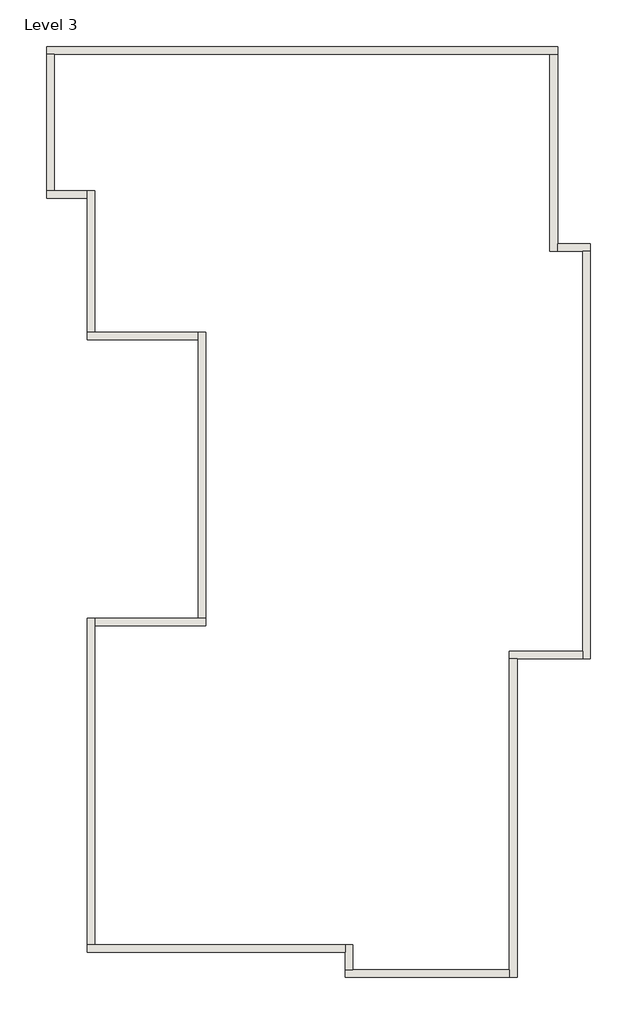
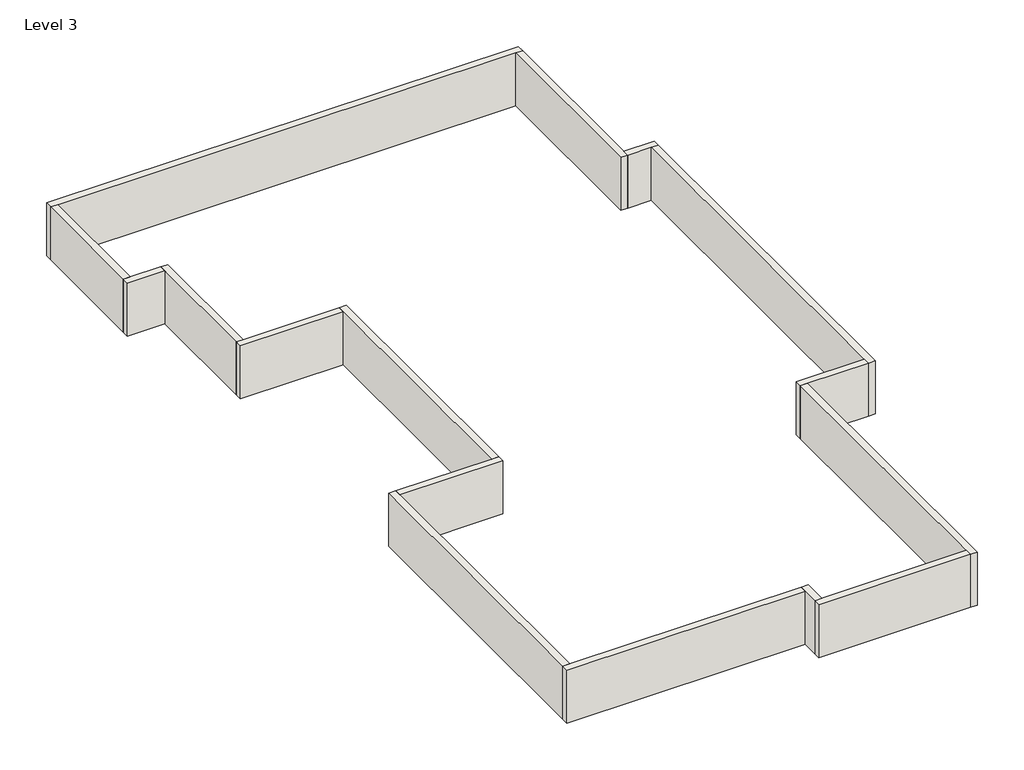
# One storey: 16 walls.
"""IFC4 building model written with IfcOpenShell, lengths in millimetres."""

from ifc_helpers import new_model, si_unit, frame, origin, place, context, project, spatial, polyline, outline, extrude, faceted_brep, element, save

model = new_model("IFC4")

# Units and contexts
model_context = context("Model", 3, world=origin())
ifc_project = project(units=[si_unit("LENGTHUNIT", "METRE", prefix="MILLI")], contexts=[model_context])

# Site, building, storey
site = spatial("IfcSite", under=ifc_project)
building = spatial("IfcBuilding", under=site)
storey = spatial("IfcBuildingStorey", under=building, Name="Level 3", Elevation=6096.0)

# Walls
placement = place(None, origin())
element("IfcWall", 1, ObjectType="wall 4.5", at=placement, inside=storey, context=model_context, shape_type="Brep", body=[
    faceted_brep([(-42682.5753088, 19549.4504636, 6096.0), (-42568.2753088, 19549.4504636, 6096.0), (-35100.6753088, 19549.4504636, 6096.0), (-34986.3753088, 19549.4504636, 6096.0), (-34986.3753088, 19549.4504636, 7010.4), (-35100.6753088, 19549.4504636, 7010.4), (-42568.2753088, 19549.4504636, 7010.4), (-42682.5753088, 19549.4504636, 7010.4), (-42682.5753088, 19663.7504636, 6096.0), (-42682.5753088, 19663.7504636, 7010.4), (-34986.3753088, 19663.7504636, 7010.4), (-34986.3753088, 19663.7504636, 6096.0)], [[[0, 1, 2, 3, 4, 5, 6, 7]], [[8, 9, 10, 11]], [[3, 2, 1, 0, 8, 11]], [[7, 6, 5, 4, 10, 9]], [[4, 3, 11, 10]], [[0, 7, 9, 8]]]),
])
element("IfcWall", 2, ObjectType="wall 4.5", at=placement, inside=storey, context=model_context, shape_type="Brep", body=[
    faceted_brep([(-35100.6753088, 19549.4504636, 6096.0), (-35100.6753088, 16577.6504636, 6096.0), (-35100.6753088, 16577.6504636, 7010.4), (-35100.6753088, 19549.4504636, 7010.4), (-34986.3753088, 19549.4504636, 6096.0), (-34986.3753088, 19549.4504636, 7010.4), (-34986.3753088, 16691.9504636, 7010.4), (-34986.3753088, 16577.6504636, 7010.4), (-34986.3753088, 16577.6504636, 6096.0), (-34986.3753088, 16691.9504636, 6096.0)], [[[0, 1, 2, 3]], [[4, 5, 6, 7, 8, 9]], [[1, 0, 4, 9, 8]], [[3, 2, 7, 6, 5]], [[0, 3, 5, 4]], [[2, 1, 8, 7]]]),
])
element("IfcWall", 3, ObjectType="wall 4.5", at=placement, inside=storey, context=model_context, shape_type="Brep", body=[
    faceted_brep([(-34986.3753088, 16577.6504636, 6096.0), (-34605.3753088, 16577.6504636, 6096.0), (-34491.0753088, 16577.6504636, 6096.0), (-34491.0753088, 16577.6504636, 7010.4), (-34605.3753088, 16577.6504636, 7010.4), (-34986.3753088, 16577.6504636, 7010.4), (-34986.3753088, 16691.9504636, 6096.0), (-34986.3753088, 16691.9504636, 7010.4), (-34491.0753088, 16691.9504636, 7010.4), (-34491.0753088, 16691.9504636, 6096.0)], [[[0, 1, 2, 3, 4, 5]], [[6, 7, 8, 9]], [[2, 1, 0, 6, 9]], [[5, 4, 3, 8, 7]], [[0, 5, 7, 6]], [[3, 2, 9, 8]]]),
])
element("IfcWall", 4, ObjectType="wall 4.5", at=placement, inside=storey, context=model_context, shape_type="Brep", body=[
    faceted_brep([(-34605.3753088, 16577.6504636, 6096.0), (-34605.3753088, 10557.8504636, 6096.0), (-34605.3753088, 10443.5504636, 6096.0), (-34605.3753088, 10443.5504636, 7010.4), (-34605.3753088, 10557.8504636, 7010.4), (-34605.3753088, 16577.6504636, 7010.4), (-34491.0753088, 16577.6504636, 6096.0), (-34491.0753088, 16577.6504636, 7010.4), (-34491.0753088, 10443.5504636, 7010.4), (-34491.0753088, 10443.5504636, 6096.0)], [[[0, 1, 2, 3, 4, 5]], [[6, 7, 8, 9]], [[2, 1, 0, 6, 9]], [[5, 4, 3, 8, 7]], [[0, 5, 7, 6]], [[3, 2, 9, 8]]]),
])
element("IfcWall", 5, ObjectType="wall 4.5", at=placement, inside=storey, context=model_context, shape_type="Brep", body=[
    faceted_brep([(-34605.3753088, 10557.8504636, 6096.0), (-35710.2753088, 10557.8504636, 6096.0), (-35710.2753088, 10557.8504636, 7010.4), (-34605.3753088, 10557.8504636, 7010.4), (-34605.3753088, 10443.5504636, 6096.0), (-34605.3753088, 10443.5504636, 7010.4), (-35595.9753088, 10443.5504636, 7010.4), (-35710.2753088, 10443.5504636, 7010.4), (-35710.2753088, 10443.5504636, 6096.0), (-35595.9753088, 10443.5504636, 6096.0)], [[[0, 1, 2, 3]], [[4, 5, 6, 7, 8, 9]], [[1, 0, 4, 9, 8]], [[3, 2, 7, 6, 5]], [[0, 3, 5, 4]], [[2, 1, 8, 7]]]),
])
element("IfcWall", 6, ObjectType="wall 4.5", at=placement, inside=storey, context=model_context, shape_type="Brep", body=[
    faceted_brep([(-35710.2753088, 10443.5504636, 6096.0), (-35710.2753088, 5757.1720573, 6096.0), (-35710.2753088, 5642.8720573, 6096.0), (-35710.2753088, 5642.8720573, 7010.4), (-35710.2753088, 5757.1720573, 7010.4), (-35710.2753088, 10443.5504636, 7010.4), (-35595.9753088, 10443.5504636, 6096.0), (-35595.9753088, 10443.5504636, 7010.4), (-35595.9753088, 5642.8720573, 7010.4), (-35595.9753088, 5642.8720573, 6096.0)], [[[0, 1, 2, 3, 4, 5]], [[6, 7, 8, 9]], [[2, 1, 0, 6, 9]], [[5, 4, 3, 8, 7]], [[0, 5, 7, 6]], [[3, 2, 9, 8]]]),
])
element("IfcWall", 7, ObjectType="wall 4.5", at=placement, inside=storey, context=model_context, shape_type="Brep", body=[
    faceted_brep([(-35710.2753088, 5757.1720573, 6096.0), (-38072.4753088, 5757.1720573, 6096.0), (-38186.7753088, 5757.1720573, 6096.0), (-38186.7753088, 5757.1720573, 7010.4), (-38072.4753088, 5757.1720573, 7010.4), (-35710.2753088, 5757.1720573, 7010.4), (-35710.2753088, 5642.8720573, 6096.0), (-35710.2753088, 5642.8720573, 7010.4), (-38186.7753088, 5642.8720573, 7010.4), (-38186.7753088, 5642.8720573, 6096.0)], [[[0, 1, 2, 3, 4, 5]], [[6, 7, 8, 9]], [[2, 1, 0, 6, 9]], [[5, 4, 3, 8, 7]], [[0, 5, 7, 6]], [[3, 2, 9, 8]]]),
])
element("IfcWall", 8, ObjectType="wall 4.5", at=placement, inside=storey, context=model_context, shape_type="Brep", body=[
    faceted_brep([(-38072.4753088, 5757.1720573, 6096.0), (-38072.4753088, 6138.2504636, 6096.0), (-38072.4753088, 6138.2504636, 7010.4), (-38072.4753088, 5757.1720573, 7010.4), (-38186.7753088, 5757.1720573, 6096.0), (-38186.7753088, 5757.1720573, 7010.4), (-38186.7753088, 6023.9504636, 7010.4), (-38186.7753088, 6138.2504636, 7010.4), (-38186.7753088, 6138.2504636, 6096.0), (-38186.7753088, 6023.9504636, 6096.0)], [[[0, 1, 2, 3]], [[4, 5, 6, 7, 8, 9]], [[1, 0, 4, 9, 8]], [[3, 2, 7, 6, 5]], [[0, 3, 5, 4]], [[2, 1, 8, 7]]]),
])
element("IfcWall", 9, ObjectType="wall 4.5", at=placement, inside=storey, context=model_context, shape_type="Brep", body=[
    faceted_brep([(-38186.7753088, 6138.2504636, 6096.0), (-41958.6753088, 6138.2504636, 6096.0), (-42072.9753088, 6138.2504636, 6096.0), (-42072.9753088, 6138.2504636, 7010.4), (-41958.6753088, 6138.2504636, 7010.4), (-38186.7753088, 6138.2504636, 7010.4), (-38186.7753088, 6023.9504636, 6096.0), (-38186.7753088, 6023.9504636, 7010.4), (-42072.9753088, 6023.9504636, 7010.4), (-42072.9753088, 6023.9504636, 6096.0)], [[[0, 1, 2, 3, 4, 5]], [[6, 7, 8, 9]], [[2, 1, 0, 6, 9]], [[5, 4, 3, 8, 7]], [[0, 5, 7, 6]], [[3, 2, 9, 8]]]),
])
element("IfcWall", 10, ObjectType="wall 4.5", at=placement, inside=storey, context=model_context, shape_type="Brep", body=[
    faceted_brep([(-41958.6753088, 6138.2504636, 6096.0), (-41958.6753088, 10938.8504636, 6096.0), (-41958.6753088, 11053.1504636, 6096.0), (-41958.6753088, 11053.1504636, 7010.4), (-41958.6753088, 10938.8504636, 7010.4), (-41958.6753088, 6138.2504636, 7010.4), (-42072.9753088, 6138.2504636, 6096.0), (-42072.9753088, 6138.2504636, 7010.4), (-42072.9753088, 11053.1504636, 7010.4), (-42072.9753088, 11053.1504636, 6096.0)], [[[0, 1, 2, 3, 4, 5]], [[6, 7, 8, 9]], [[2, 1, 0, 6, 9]], [[5, 4, 3, 8, 7]], [[0, 5, 7, 6]], [[3, 2, 9, 8]]]),
])
element("IfcWall", 11, ObjectType="wall 4.5", at=placement, inside=storey, context=model_context, shape_type="Brep", body=[
    faceted_brep([(-41958.6753088, 10938.8504636, 6096.0), (-40281.7832488, 10938.8504636, 6096.0), (-40281.7832488, 10938.8504636, 7010.4), (-41958.6753088, 10938.8504636, 7010.4), (-41958.6753088, 11053.1504636, 6096.0), (-41958.6753088, 11053.1504636, 7010.4), (-40396.0832488, 11053.1504636, 7010.4), (-40281.7832488, 11053.1504636, 7010.4), (-40281.7832488, 11053.1504636, 6096.0), (-40396.0832488, 11053.1504636, 6096.0)], [[[0, 1, 2, 3]], [[4, 5, 6, 7, 8, 9]], [[1, 0, 4, 9, 8]], [[3, 2, 7, 6, 5]], [[0, 3, 5, 4]], [[2, 1, 8, 7]]]),
])
element("IfcWall", 12, ObjectType="wall 4.5", at=placement, inside=storey, context=model_context, shape_type="Brep", body=[
    faceted_brep([(-40281.7832488, 11053.1504636, 6096.0), (-40281.7832488, 15358.4504636, 6096.0), (-40281.7832488, 15358.4504636, 7010.4), (-40281.7832488, 11053.1504636, 7010.4), (-40396.0832488, 11053.1504636, 6096.0), (-40396.0832488, 11053.1504636, 7010.4), (-40396.0832488, 15244.1504636, 7010.4), (-40396.0832488, 15358.4504636, 7010.4), (-40396.0832488, 15358.4504636, 6096.0), (-40396.0832488, 15244.1504636, 6096.0)], [[[0, 1, 2, 3]], [[4, 5, 6, 7, 8, 9]], [[1, 0, 4, 9, 8]], [[3, 2, 7, 6, 5]], [[0, 3, 5, 4]], [[2, 1, 8, 7]]]),
])
element("IfcWall", 13, ObjectType="wall 4.5", at=placement, inside=storey, context=model_context, shape_type="Brep", body=[
    faceted_brep([(-40396.0832488, 15358.4504636, 6096.0), (-41958.6753088, 15358.4504636, 6096.0), (-42072.9753088, 15358.4504636, 6096.0), (-42072.9753088, 15358.4504636, 7010.4), (-41958.6753088, 15358.4504636, 7010.4), (-40396.0832488, 15358.4504636, 7010.4), (-40396.0832488, 15244.1504636, 6096.0), (-40396.0832488, 15244.1504636, 7010.4), (-42072.9753088, 15244.1504636, 7010.4), (-42072.9753088, 15244.1504636, 6096.0)], [[[0, 1, 2, 3, 4, 5]], [[6, 7, 8, 9]], [[2, 1, 0, 6, 9]], [[5, 4, 3, 8, 7]], [[0, 5, 7, 6]], [[3, 2, 9, 8]]]),
])
element("IfcWall", 14, ObjectType="wall 4.5", at=placement, inside=storey, context=model_context, shape_type="Brep", body=[
    faceted_brep([(-41958.6753088, 15358.4504636, 6096.0), (-41958.6753088, 17492.0504636, 6096.0), (-41958.6753088, 17492.0504636, 7010.4), (-41958.6753088, 15358.4504636, 7010.4), (-42072.9753088, 15358.4504636, 6096.0), (-42072.9753088, 15358.4504636, 7010.4), (-42072.9753088, 17377.7504636, 7010.4), (-42072.9753088, 17492.0504636, 7010.4), (-42072.9753088, 17492.0504636, 6096.0), (-42072.9753088, 17377.7504636, 6096.0)], [[[0, 1, 2, 3]], [[4, 5, 6, 7, 8, 9]], [[1, 0, 4, 9, 8]], [[3, 2, 7, 6, 5]], [[0, 3, 5, 4]], [[2, 1, 8, 7]]]),
])
element("IfcWall", 15, ObjectType="wall 4.5", at=placement, inside=storey, context=model_context, shape_type="Brep", body=[
    faceted_brep([(-42072.9753088, 17492.0504636, 6096.0), (-42568.2753088, 17492.0504636, 6096.0), (-42682.5753088, 17492.0504636, 6096.0), (-42682.5753088, 17492.0504636, 7010.4), (-42568.2753088, 17492.0504636, 7010.4), (-42072.9753088, 17492.0504636, 7010.4), (-42072.9753088, 17377.7504636, 6096.0), (-42072.9753088, 17377.7504636, 7010.4), (-42682.5753088, 17377.7504636, 7010.4), (-42682.5753088, 17377.7504636, 6096.0)], [[[0, 1, 2, 3, 4, 5]], [[6, 7, 8, 9]], [[2, 1, 0, 6, 9]], [[5, 4, 3, 8, 7]], [[0, 5, 7, 6]], [[3, 2, 9, 8]]]),
])
element("IfcWall", 16, ObjectType="wall 4.5", at=placement, inside=storey, context=model_context, shape_type="SweptSolid", body=[
    extrude(outline(polyline([(-42568.2753088, 19549.4504636), (-42568.2753088, 17492.0504636), (-42682.5753088, 17492.0504636), (-42682.5753088, 19549.4504636), (-42568.2753088, 19549.4504636)])), frame((0.0, 0.0, 6096.0), z_axis=(0.0, 0.0, 1.0), x_axis=(1.0, 0.0, 0.0)), (0.0, 0.0, 1.0), 914.4),
])

save(model, "model.ifc")

# Revit data of these elements
# Type "wall 4.5"
#   Assembly Code = "B2010"
#   Layers, outside or top first: 0' - 4 1/2" no material (function 1)
# Elements 1, 2, 3, 4, 5, 6, 7, 8, 9, 10, 11, 12, 13, 14, 15, 16 (IfcWall, "wall 4.5")
#   Top Offset = 0' - 0"
#   Base Offset = 0' - 0"
#   wall height = 3' - 0"
#   Phase Created = New Construction
#   Base Constraint = Level 3
#   Top Constraint = Level 7
#   Materials on its faces: "Default Wall"
# Materials
#   "Default Wall": colour RGB 128 128 128, transparency 0, Cost = 0
